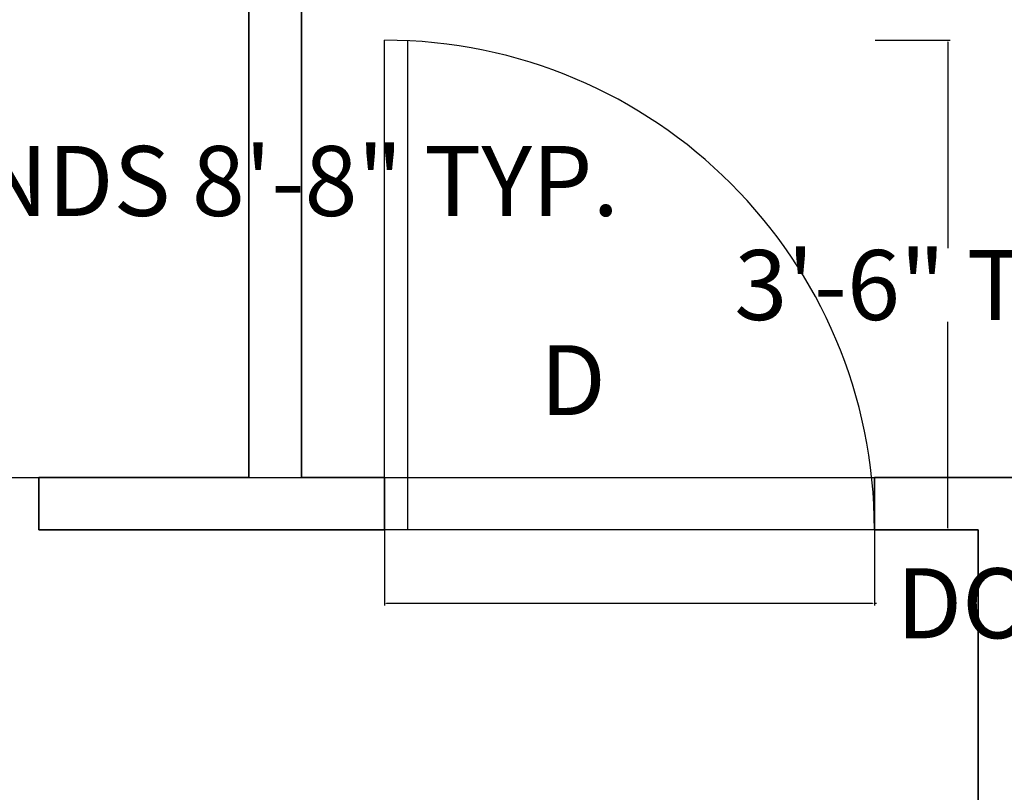
# Model space of a CAD drawing. Units: inches. Extents: x -26 to 575, y -18 to 513.
# Tile 24 of 28: x 355 to 439, y 307 to 374. Entities that reach past the tile are written whole.
import ezdxf

# ---------------------------------------------------------------- set-up
doc = ezdxf.new("R2010")
doc.units = ezdxf.units.IN
doc.header["$MEASUREMENT"] = 0
for name, color, linetype, lineweight in [('A-ANNO-DIMS', 2, 'Continuous', 18), ('A-ANNO-TEXT', 7, 'Continuous', 18), ('A-DOOR', 3, 'Continuous', 25), ('A-WALL', 7, 'Continuous', 35)]:
    doc.layers.add(name, color=color, linetype=linetype, lineweight=lineweight)
doc.styles.get("Standard").update_dxf_attribs({"font": 'arial.ttf', "height": 6})
doc.dimstyles.get("Standard").update_dxf_attribs({"dimtxt": 6, "dimasz": 0.18, "dimexe": 0.18, "dimexo": 0.0625, "dimgap": 0.09, "dimtad": 0, "dimtih": 1, "dimtoh": 1, "dimzin": 0, "dimdsep": 46, "dimlunit": 3, "dimtxsty": 'Standard', "dimcen": 0.09, "dimadec": 0, "dimazin": 0, "dimtfac": 1, "dimtofl": 0, "dimtmove": 0, "dimatfit": 3, "dimfxl": 1, "dimtolj": 1, "dimtzin": 0, "dimarcsym": 0})

# ---------------------------------------------------------------- blocks, each defined once
blk = doc.blocks.new('DOOR-SWING-42IN')
for p, q in [((0, 0), (0, 42)), ((2, 0), (2, 42)), ((42, 0), (0, 0))]:
    blk.add_line(p, q)
blk.add_arc((0, 0), 42, 0, 90)
blk = doc.blocks.new('*D12')
at = {"layer": 'A-ANNO-DIMS', "color": 0, "lineweight": -2, "transparency": 16777216}
for p, q in [((143.378, 375.468), (143.378, 359.755)), ((247.348, 375.468), (247.348, 359.755)), ((143.558, 359.935), (247.168, 359.935)), ((247.348, 359.935), (247.528, 359.935))]:
    blk.add_line(p, q, dxfattribs=at)
at = {"layer": 'A-ANNO-DIMS', "color": 0, "transparency": 16777216}
for points in [[(143.558, 359.965), (143.558, 359.905), (143.378, 359.935)], [(247.168, 359.965), (247.168, 359.905), (247.348, 359.935)]]:
    blk.add_solid(points, dxfattribs=at)
at = {"layer": 'Defpoints', "color": 0, "transparency": 16777216}
for p in [(143.378, 375.531), (247.348, 375.531), (247.348, 359.935)]:
    blk.add_point(p, dxfattribs=at)
at = {"layer": 'A-ANNO-DIMS', "color": 0, "transparency": 16777216, "insert": (329.097, 359.935), "char_height": 6, "attachment_point": 5}
blk.add_mtext('\\A1;DOUBLE BED & NIGHTSTANDS 8\'-8" TYP.', dxfattribs=at)
blk = doc.blocks.new('*D14')
at = {"layer": 'A-ANNO-DIMS', "color": 0, "lineweight": -2, "transparency": 16777216}
for p, q in [((385.797, 329.945), (385.797, 323.528)), ((427.797, 329.945), (427.797, 323.528)), ((385.977, 323.708), (427.617, 323.708)), ((427.797, 323.708), (427.977, 323.708))]:
    blk.add_line(p, q, dxfattribs=at)
at = {"layer": 'A-ANNO-DIMS', "color": 0, "transparency": 16777216}
for points in [[(385.977, 323.738), (385.977, 323.678), (385.797, 323.708)], [(427.617, 323.738), (427.617, 323.678), (427.797, 323.708)]]:
    blk.add_solid(points, dxfattribs=at)
at = {"layer": 'Defpoints', "color": 0, "transparency": 16777216}
for p in [(385.797, 330.008), (427.797, 330.008), (427.797, 323.708)]:
    blk.add_point(p, dxfattribs=at)
at = {"layer": 'A-ANNO-DIMS', "color": 0, "transparency": 16777216, "insert": (464.132, 323.708), "char_height": 6, "attachment_point": 5}
blk.add_mtext('\\A1;DOOR D 3\'-6" TYP.', dxfattribs=at)
blk = doc.blocks.new('*D15')
at = {"layer": 'A-ANNO-DIMS', "color": 0, "lineweight": -2, "transparency": 16777216}
for p, q in [((427.859, 372.008), (434.277, 372.008)), ((434.097, 371.828), (434.097, 354.163)), ((434.097, 330.188), (434.097, 347.853)), ((427.859, 330.008), (434.277, 330.008))]:
    blk.add_line(p, q, dxfattribs=at)
at = {"layer": 'A-ANNO-DIMS', "color": 0, "transparency": 16777216}
for points in [[(434.067, 371.828), (434.127, 371.828), (434.097, 372.008)], [(434.067, 330.188), (434.127, 330.188), (434.097, 330.008)]]:
    blk.add_solid(points, dxfattribs=at)
at = {"layer": 'Defpoints', "color": 0, "transparency": 16777216}
for p in [(427.797, 372.008), (434.097, 372.008), (427.797, 330.008)]:
    blk.add_point(p, dxfattribs=at)
at = {"layer": 'A-ANNO-DIMS', "color": 0, "transparency": 16777216, "insert": (434.097, 351.008), "char_height": 6, "attachment_point": 5}
blk.add_mtext('\\A1;3\'-6" TYP.', dxfattribs=at)
blk = doc.blocks.new('*D31')
at = {"layer": 'A-ANNO-DIMS', "color": 0, "lineweight": -2, "transparency": 16777216}
for p, q in [((311.292, 466.445), (311.292, -8.972)), ((336.72, 466.445), (336.72, -8.972)), ((311.472, -8.792), (336.54, -8.792)), ((336.72, -8.792), (336.9, -8.792))]:
    blk.add_line(p, q, dxfattribs=at)
at = {"layer": 'A-ANNO-DIMS', "color": 0, "transparency": 16777216}
for points in [[(311.472, -8.762), (311.472, -8.822), (311.292, -8.792)], [(336.54, -8.762), (336.54, -8.822), (336.72, -8.792)]]:
    blk.add_solid(points, dxfattribs=at)
at = {"layer": 'Defpoints', "color": 0, "transparency": 16777216}
for p in [(311.292, 466.508), (336.72, 466.508), (336.72, -8.792)]:
    blk.add_point(p, dxfattribs=at)
at = {"layer": 'A-ANNO-DIMS', "color": 0, "transparency": 16777216, "insert": (352.006, -8.792), "char_height": 6, "attachment_point": 5}
blk.add_mtext('\\A1;2\'-1 1/2"', dxfattribs=at)
blk = doc.blocks.new('*D49')
at = {"layer": 'A-ANNO-DIMS', "color": 0, "lineweight": -2, "transparency": 16777216}
for p, q in [((278.24, 466.508), (550.657, 466.508)), ((550.477, 466.328), (550.477, 403.661)), ((550.477, 334.688), (550.477, 397.355)), ((278.24, 334.508), (550.657, 334.508))]:
    blk.add_line(p, q, dxfattribs=at)
at = {"layer": 'A-ANNO-DIMS', "color": 0, "transparency": 16777216}
for points in [[(550.447, 466.328), (550.507, 466.328), (550.477, 466.508)], [(550.447, 334.688), (550.507, 334.688), (550.477, 334.508)]]:
    blk.add_solid(points, dxfattribs=at)
at = {"layer": 'Defpoints', "color": 0, "transparency": 16777216}
for p in [(278.177, 466.508), (550.477, 466.508), (278.177, 334.508)]:
    blk.add_point(p, dxfattribs=at)
at = {"layer": 'A-ANNO-DIMS', "color": 0, "transparency": 16777216, "insert": (550.477, 400.508), "char_height": 6, "attachment_point": 5}
blk.add_mtext('\\A1;11\'-0"', dxfattribs=at)

msp = doc.modelspace()

# ---------------------------------------------------------------- linework, layer by layer
at = {"layer": 'A-WALL'}
for p, q in [((374.177, 334.508), (374.177, 466.508)), ((378.677, 334.508), (378.677, 466.508)), ((374.177, 334.508), (356.177, 334.508)), ((356.177, 334.508), (356.177, 330.008)), ((385.797, 334.508), (378.677, 334.508)), ((385.797, 334.508), (385.797, 330.008)), ((427.797, 334.508), (427.797, 330.008)), ((471.534, 334.508), (427.797, 334.508)), ((374.177, 330.008), (356.177, 330.008)), ((385.797, 330.008), (374.177, 330.008)), ((436.677, 330.008), (427.797, 330.008)), ((436.677, 298.508), (436.677, 330.008))]:
    msp.add_line(p, q, dxfattribs=at)

# ---------------------------------------------------------------- block references
at = {"layer": 'A-DOOR'}
msp.add_blockref('DOOR-SWING-42IN', (385.797, 330.008), dxfattribs=at)

# ---------------------------------------------------------------- texts
at = {"layer": 'A-ANNO-TEXT'}
msp.add_text('D', height=6, rotation=0.00167, dxfattribs=at).set_placement((399.138, 339.849))

# ---------------------------------------------------------------- dimensions: what is measured, and where the dimension line sits
at = {"layer": 'A-ANNO-DIMS'}
dim = msp.add_linear_dim(base=(550.477, 466.508), p1=(278.177, 334.508), p2=(278.177, 466.508), angle=90, dimstyle='Standard', override={"dimdec": 1, "dimlfac": 1, "dimrnd": 0, "dimzin": 1, "dimdsep": 46, "dimlunit": 4, "dimfrac": 2}, dxfattribs=at)
dim.commit()
dim.dimension.update_dxf_attribs({"geometry": '*D49', "text_midpoint": (550.477, 400.508)})
dim = msp.add_linear_dim(base=(336.72, -8.792), p1=(311.292, 466.508), p2=(336.72, 466.508), dimstyle='Standard', override={"dimdec": 1, "dimlfac": 1, "dimrnd": 0, "dimzin": 1, "dimdsep": 46, "dimlunit": 4, "dimfrac": 2}, dxfattribs=at)
dim.commit()
dim.dimension.update_dxf_attribs({"geometry": '*D31', "text_midpoint": (352.006, -8.792)})
for base, p1, p2, text, picture, middle in [((247.348, 359.935), (143.378, 375.531), (247.348, 375.531), 'DOUBLE BED & NIGHTSTANDS <> TYP.', '*D12', (329.097, 359.935)), ((427.797, 323.708), (385.797, 330.008), (427.797, 330.008), 'DOOR D <> TYP.', '*D14', (464.132, 323.708))]:
    dim = msp.add_linear_dim(base=base, p1=p1, p2=p2, text=text, dimstyle='Standard', override={"dimdec": 1, "dimlfac": 1, "dimrnd": 0, "dimzin": 1, "dimdsep": 46, "dimlunit": 4, "dimfrac": 2}, dxfattribs=at)
    dim.commit()
    dim.dimension.update_dxf_attribs({"geometry": picture, "text_midpoint": middle})
dim = msp.add_linear_dim(base=(434.097, 372.008), p1=(427.797, 330.008), p2=(427.797, 372.008), angle=90, text='<> TYP.', dimstyle='Standard', override={"dimdec": 1, "dimlfac": 1, "dimrnd": 0, "dimzin": 1, "dimdsep": 46, "dimlunit": 4, "dimfrac": 2}, dxfattribs=at)
dim.commit()
dim.dimension.update_dxf_attribs({"geometry": '*D15', "text_midpoint": (434.097, 351.008)})

doc.saveas('drawing.dxf')
